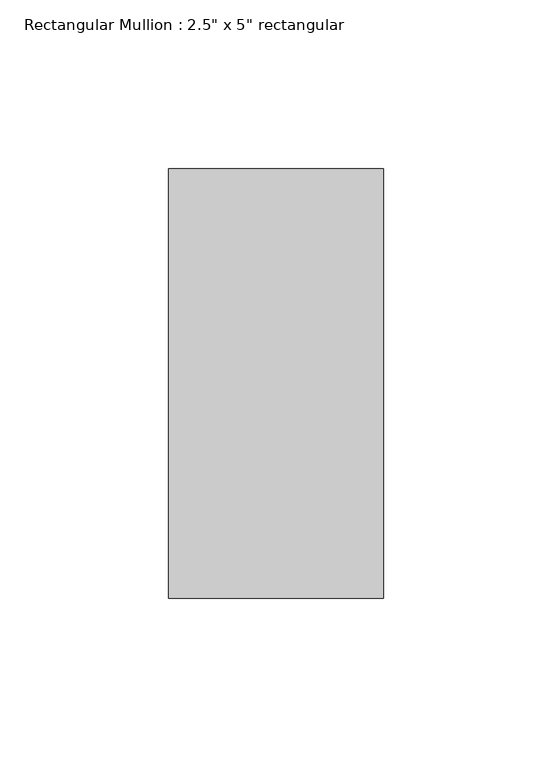
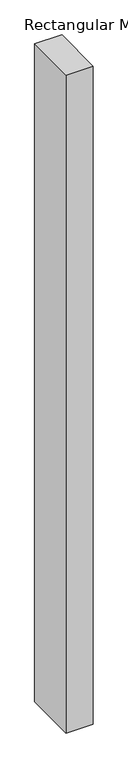
"""IFC4 building model written with IfcOpenShell, lengths in millimetres: member geometry."""

from ifc_helpers import new_model, si_unit, frame, origin, place, context, project, spatial, polyline, outline, extrude, source, transform, mapped, element, save


def member_7a2ba7d2(model_context):
    return source(origin(), model_context, "Body", "SweptSolid", [
        extrude(outline(polyline([(0.0, 63.5), (0.0, -63.5), (-63.5, -63.5), (-63.5, 63.5), (0.0, 63.5)])), frame((0.0, 0.0, -1624.4964589), z_axis=(0.0, 0.0, 1.0), x_axis=(1.0, 0.0, 0.0)), (0.0, 0.0, 1.0), 1624.4964589),
    ])


if __name__ == "__main__":
    model = new_model("IFC4")
    model_context = context("Model", 3, world=origin())
    ifc_project = project(units=[si_unit("LENGTHUNIT", "METRE", prefix="MILLI")], contexts=[model_context])
    site = spatial("IfcSite", under=ifc_project)
    building = spatial("IfcBuilding", under=site)
    placement = place(None, origin())
    member_shape = member_7a2ba7d2(model_context)
    element("IfcMember", 1, ObjectType="Rectangular Mullion : 2.5\" x 5\" rectangular", at=placement, inside=building, context=model_context, shape_type="MappedRepresentation", body=[
        mapped(member_shape, transform((0.0, 0.0, 0.0), x_axis=(1.0, 0.0, 0.0), y_axis=(0.0, 1.0, 0.0), z_axis=(0.0, 0.0, 1.0))),
    ])
    save(model, "model.ifc")

# Revit data of these elements
# Type "Rectangular Mullion : 2.5\" x 5\" rectangular"
#   built-in parameter 1007304 = 0.416667 (stored number, unit not read)
#   built-in parameter 1007301 = 0.104167 (stored number, unit not read)
#   built-in parameter 1007300 = 0.104167 (stored number, unit not read)
# Element 1 (IfcMember, "Rectangular Mullion : 2.5\" x 5\" rectangular")
#   Materials on its faces: "Aluminum"
# Materials
#   "Aluminum": class "Metal", colour RGB 247 247 247, transparency 0, Description = "Aluminum 6061", Cost = 0
